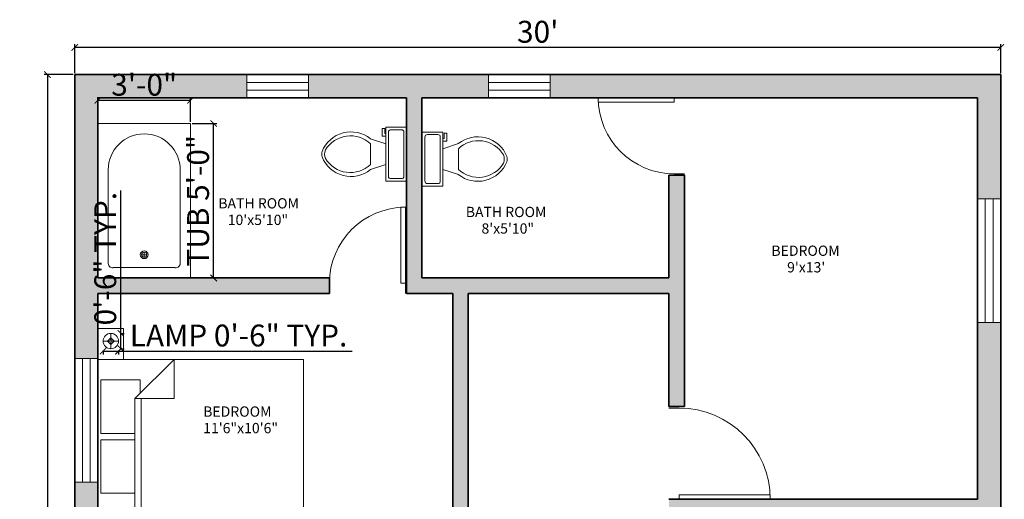
# Model space of a CAD drawing. Units: inches. Extents: x 3799 to 20199, y 1682 to 8087.
# Tile 17 of 30: x 10500 to 10883, y 7631 to 7817. Entities that reach past the tile are written whole.
import ezdxf

# ---------------------------------------------------------------- set-up
doc = ezdxf.new("R2010")
doc.units = ezdxf.units.IN
for name, color, linetype, lineweight in [('A-ANNO-DIMS', 2, 'Continuous', 18), ('A-AREA-IDEN', 7, 'Continuous', 18), ('A-DOOR', 3, 'Continuous', 18), ('A-FLOR-FIXT', 9, 'Continuous', 18), ('A-FURN', 8, 'Continuous', 18), ('A-GLAZ', 152, 'Continuous', 18), ('A-WALL', 7, 'Continuous', 35), ('A-WALL-PATT', 252, 'Continuous', 13)]:
    doc.layers.add(name, color=color, linetype=linetype, lineweight=lineweight)
doc.styles.get("Standard").update_dxf_attribs({"font": 'arial.ttf'})
doc.dimstyles.new('ISO-25', dxfattribs={"dimtxt": 8.5, "dimasz": 2.5, "dimexe": 1.25, "dimexo": 0.625, "dimtad": 1, "dimdec": 0, "dimlunit": 3, "dimtxsty": 'Standard', "dimblk": 'ARCHTICK', "dimcen": 2.5, "dimadec": 0, "dimazin": 0, "dimtfac": 1, "dimtdec": 0, "dimtmove": 0, "dimatfit": 3, "dimfxl": 1, "dimarcsym": 0})

# ---------------------------------------------------------------- blocks, each defined once
blk = doc.blocks.new('*U48')
for p, q in [((-750, 0), (-750, -100)), ((0, 0), (0, -100))]:
    blk.add_line(p, q)
blk.add_lwpolyline([(0, 0), (0, 750), (-43.75, 750), (-43.75, 0)], close=True)
blk.add_arc((0, 0), 750, 90, 180)
blk = doc.blocks.new('*U124')
for p, q in [((0, 0), (0, -100)), ((-900, 0), (-900, -100))]:
    blk.add_line(p, q)
blk.add_lwpolyline([(0, 0), (0, 900), (-43.75, 900), (-43.75, 0)], close=True)
blk.add_arc((0, 0), 900, 90, 180)
blk = doc.blocks.new('Bed - Queen')
for p, q in [((0, -80.00003), (0, 0)), ((0, 0), (59.99999, 0)), ((59.99999, 0), (59.99999, -80.00003)), ((7.99999, -1.2), (28.79998, -1.2)), ((7.99999, -14.4), (7.99999, -1.2)), ((28.79998, -1.2), (28.79998, -14.4)), ((31.19999, -1.2), (51.99999, -1.2)), ((31.19999, -14.4), (31.19999, -1.2)), ((51.99999, -1.2), (51.99999, -16.4)), ((0, -14.4), (44.8, -14.4)), ((59.99999, -29.6), (44.8, -14.4)), ((44.8, -14.4), (44.8, -29.6)), ((44.8, -16.8), (0, -16.8)), ((51.99999, -16.4), (46.79936, -16.4)), ((44.8, -29.6), (59.99999, -29.6)), ((59.99999, -80.00003), (0, -80.00003))]:
    blk.add_line(p, q)
blk = doc.blocks.new('Lamp - Table')
for p, q in [((-1, 0), (-7, 0)), ((0, 3), (-3, 0)), ((-3, 0), (0, -3)), ((0, 7), (0, 1)), ((3, 0), (0, 3)), ((0, -3), (3, 0)), ((1, 0), (7, 0)), ((0, -1), (0, -7))]:
    blk.add_line(p, q)
for radius in [7, 1]:
    blk.add_circle((0, 0), radius)
blk = doc.blocks.new('Bath Tub - 26 x 60 in.')
for p, q in [((8, -18), (10, -18)), ((9, -17), (9, -19))]:
    blk.add_line(p, q)
blk.add_lwpolyline([(0, -36), (0, 0), (60, 0), (60, -36)], close=True)
for points in [[(4, -30), (4, -6)], [(6, -4), (42, -4)], [(42, -32), (6, -32)]]:
    blk.add_lwpolyline(points)
for radius in [1.5, 1]:
    blk.add_circle((9, -18), radius)
for centre, radius, start, end in [((5.75, -5.75), 1.77, 81.8699, 188.1301), ((42, -18), 14, 270, 90), ((5.75, -30.25), 1.77, 171.8699, 278.1301)]:
    blk.add_arc(centre, radius, start, end)
blk = doc.blocks.new('Toilet - top')
for p, q in [((9.5, -6), (9.5, -2)), ((-10, -8.5), (-8, -8.5)), ((-10, -9.5), (-10, -8.5)), ((-7, -9.5), (-10, -9.5)), ((-8, -8.5), (-8, -8)), ((-7, -8), (-7, -9.5)), ((-4, -8), (-6, -14)), ((4, -8), (6, -14)), ((4, -14), (-4, -14))]:
    blk.add_line(p, q)
blk.add_lwpolyline([(10.5, -8), (10.5, 0), (-10.5, 0), (-10.5, -8)], close=True)
for points in [[(-9.5, -2), (-9.5, -6)], [(8.5, -1), (-8.5, -1)], [(-8.5, -7), (8.5, -7)]]:
    blk.add_lwpolyline(points)
for centre, radius, start, end in [((-8.62, -1.88), 0.884, 81.8699, 188.1301), ((8.62, -1.88), 0.884, 351.8699, 98.1301), ((-8.62, -6.12), 0.884, 171.8699, 278.1301), ((8.62, -6.12), 0.884, 261.8699, 8.1301), ((3.52, -21.58), 12.17, 141.4691, 247.9714), ((4.2, -21.82), 11.33, 136.3677, 238.9468), ((-3.52, -21.58), 12.17, 292.0284, 38.5307), ((-4.2, -21.82), 11.33, 301.053, 43.6321), ((0, -27.88), 4, 245.7318, 294.2682), ((0, -29), 4, 254.8605, 285.1395)]:
    blk.add_arc(centre, radius, start, end)
blk = doc.blocks.new('_ArchTick')
at = {"color": 0, "linetype": 'ByBlock', "const_width": 0.15}
blk.add_lwpolyline([(-0.5, -0.5), (0.5, 0.5)], dxfattribs=at)
blk = doc.blocks.new('*D175')
at = {"layer": 'A-ANNO-DIMS', "color": 0, "lineweight": -2, "transparency": 16777216}
for p, q in [((10521.87, 7796.25), (10521.87, 7807.45)), ((10881.87, 7806.2), (10521.87, 7806.2)), ((10881.87, 7796.25), (10881.87, 7807.45))]:
    blk.add_line(p, q, dxfattribs=at)
at = {"layer": 'Defpoints', "color": 0, "transparency": 16777216}
for p in [(10521.87, 7806.2), (10521.87, 7795.62), (10881.87, 7795.62)]:
    blk.add_point(p, dxfattribs=at)
at = {"layer": 'A-ANNO-DIMS', "color": 0, "lineweight": -2, "transparency": 16777216, "xscale": 2.5, "yscale": 2.5, "zscale": 2.5, "rotation": 180}
blk.add_blockref('_ArchTick', (10521.87, 7806.2), dxfattribs=at)
at = {"layer": 'A-ANNO-DIMS', "color": 0, "lineweight": -2, "transparency": 16777216, "xscale": 2.5, "yscale": 2.5, "zscale": 2.5}
blk.add_blockref('_ArchTick', (10881.87, 7806.2), dxfattribs=at)
at = {"layer": 'A-ANNO-DIMS', "color": 0, "transparency": 16777216, "insert": (10701.87, 7811.17), "char_height": 8.5, "attachment_point": 5}
blk.add_mtext("30'", dxfattribs=at)
blk = doc.blocks.new('*D176')
at = {"layer": 'A-ANNO-DIMS', "color": 0, "lineweight": -2, "transparency": 16777216}
for p, q in [((10521.25, 7795.62), (10509.98, 7795.62)), ((10511.23, 7795.62), (10511.23, 7315.62)), ((10521.25, 7315.62), (10509.98, 7315.62))]:
    blk.add_line(p, q, dxfattribs=at)
at = {"layer": 'Defpoints', "color": 0, "transparency": 16777216}
for p in [(10521.87, 7795.62), (10511.23, 7315.62), (10521.87, 7315.62)]:
    blk.add_point(p, dxfattribs=at)
at = {"layer": 'A-ANNO-DIMS', "color": 0, "lineweight": -2, "transparency": 16777216, "xscale": 2.5, "yscale": 2.5, "zscale": 2.5}
for p, rotation in [((10511.23, 7795.62), 90), ((10511.23, 7315.62), 270)]:
    blk.add_blockref('_ArchTick', p, dxfattribs=dict(at, rotation=rotation))
at = {"layer": 'A-ANNO-DIMS', "color": 0, "transparency": 16777216, "insert": (10506.27, 7555.62), "char_height": 8.5, "attachment_point": 5, "rotation": 90}
blk.add_mtext("40'", dxfattribs=at)
blk = doc.blocks.new('WIN-24IN-9IN-FRAME')
for p, q in [((0, 24), (9, 24)), ((3, 0), (3, 24)), ((6, 0), (6, 24)), ((0, 0), (9, 0))]:
    blk.add_line(p, q)
blk = doc.blocks.new('WIN-48IN-9IN-FRAME')
for p, q in [((0, 0), (0, 9)), ((48, 0), (48, 9)), ((48, 6), (0, 6)), ((48, 3), (0, 3))]:
    blk.add_line(p, q)
blk = doc.blocks.new('*D250')
at = {"layer": 'A-ANNO-DIMS', "color": 0, "lineweight": -2, "transparency": 16777216}
for p, q in [((10532.9, 7688.46), (10532.9, 7686.94)), ((10532.9, 7688.19), (10538.9, 7688.19)), ((10538.9, 7688.46), (10538.9, 7686.94)), ((10538.9, 7688.19), (10629.72, 7688.19))]:
    blk.add_line(p, q, dxfattribs=at)
at = {"layer": 'Defpoints', "color": 0, "transparency": 16777216}
for p in [(10532.9, 7689.09), (10538.9, 7689.09), (10538.9, 7688.19)]:
    blk.add_point(p, dxfattribs=at)
at = {"layer": 'A-ANNO-DIMS', "color": 0, "lineweight": -2, "transparency": 16777216, "xscale": 2.5, "yscale": 2.5, "zscale": 2.5, "rotation": 180}
blk.add_blockref('_ArchTick', (10532.9, 7688.19), dxfattribs=at)
at = {"layer": 'A-ANNO-DIMS', "color": 0, "lineweight": -2, "transparency": 16777216, "xscale": 2.5, "yscale": 2.5, "zscale": 2.5}
blk.add_blockref('_ArchTick', (10538.9, 7688.19), dxfattribs=at)
at = {"layer": 'A-ANNO-DIMS', "color": 0, "transparency": 16777216, "insert": (10585.56, 7693.15), "char_height": 8.5, "attachment_point": 5}
blk.add_mtext('LAMP 0\'-6" TYP.', dxfattribs=at)
blk = doc.blocks.new('*D251')
at = {"layer": 'A-ANNO-DIMS', "color": 0, "lineweight": -2, "transparency": 16777216}
for p, q in [((10539.8, 7695.09), (10539.8, 7750.65)), ((10539.52, 7695.09), (10541.05, 7695.09)), ((10539.8, 7689.09), (10539.8, 7695.09)), ((10539.52, 7689.09), (10541.05, 7689.09))]:
    blk.add_line(p, q, dxfattribs=at)
at = {"layer": 'Defpoints', "color": 0, "transparency": 16777216}
for p in [(10538.9, 7695.09), (10539.8, 7695.09), (10538.9, 7689.09)]:
    blk.add_point(p, dxfattribs=at)
at = {"layer": 'A-ANNO-DIMS', "color": 0, "lineweight": -2, "transparency": 16777216, "xscale": 2.5, "yscale": 2.5, "zscale": 2.5}
for p, rotation in [((10539.8, 7695.09), 90), ((10539.8, 7689.09), 270)]:
    blk.add_blockref('_ArchTick', p, dxfattribs=dict(at, rotation=rotation))
at = {"layer": 'A-ANNO-DIMS', "color": 0, "transparency": 16777216, "insert": (10534.83, 7724.12), "char_height": 8.5, "attachment_point": 5, "rotation": 90}
blk.add_mtext('0\'-6" TYP.', dxfattribs=at)
blk = doc.blocks.new('*D308')
at = {"layer": 'A-ANNO-DIMS', "color": 0, "lineweight": -2, "transparency": 16777216}
for p, q in [((10567.5, 7776.62), (10577.12, 7776.62)), ((10575.87, 7716.62), (10575.87, 7776.62)), ((10567.5, 7716.62), (10577.12, 7716.62))]:
    blk.add_line(p, q, dxfattribs=at)
at = {"layer": 'Defpoints', "color": 0, "transparency": 16777216}
for p in [(10566.87, 7776.62), (10575.87, 7776.62), (10566.87, 7716.62)]:
    blk.add_point(p, dxfattribs=at)
at = {"layer": 'A-ANNO-DIMS', "color": 0, "lineweight": -2, "transparency": 16777216, "xscale": 2.5, "yscale": 2.5, "zscale": 2.5}
for p, rotation in [((10575.87, 7776.62), 90), ((10575.87, 7716.62), 270)]:
    blk.add_blockref('_ArchTick', p, dxfattribs=dict(at, rotation=rotation))
at = {"layer": 'A-ANNO-DIMS', "color": 0, "transparency": 16777216, "insert": (10570.91, 7746.62), "char_height": 8.5, "attachment_point": 5, "rotation": 90}
blk.add_mtext('TUB 5\'-0"', dxfattribs=at)
blk = doc.blocks.new('*D309')
at = {"layer": 'A-ANNO-DIMS', "color": 0, "lineweight": -2, "transparency": 16777216}
for p, q in [((10530.87, 7777.25), (10530.87, 7786.87)), ((10566.87, 7777.25), (10566.87, 7786.87)), ((10566.87, 7785.62), (10530.87, 7785.62))]:
    blk.add_line(p, q, dxfattribs=at)
at = {"layer": 'Defpoints', "color": 0, "transparency": 16777216}
for p in [(10530.87, 7785.62), (10530.87, 7776.62), (10566.87, 7776.62)]:
    blk.add_point(p, dxfattribs=at)
at = {"layer": 'A-ANNO-DIMS', "color": 0, "lineweight": -2, "transparency": 16777216, "xscale": 2.5, "yscale": 2.5, "zscale": 2.5, "rotation": 180}
blk.add_blockref('_ArchTick', (10530.87, 7785.62), dxfattribs=at)
at = {"layer": 'A-ANNO-DIMS', "color": 0, "lineweight": -2, "transparency": 16777216, "xscale": 2.5, "yscale": 2.5, "zscale": 2.5}
blk.add_blockref('_ArchTick', (10566.87, 7785.62), dxfattribs=at)
at = {"layer": 'A-ANNO-DIMS', "color": 0, "transparency": 16777216, "insert": (10548.87, 7790.59), "char_height": 8.5, "attachment_point": 5}
blk.add_mtext('3\'-0"', dxfattribs=at)

msp = doc.modelspace()

# ---------------------------------------------------------------- hatches: boundary and pattern name
at = {"layer": 'A-WALL-PATT'}
h = msp.add_hatch(color=256, dxfattribs=at)
h.dxf.hatch_style = 1
h.paths.add_polyline_path([(10588.75, 7795.62), (10521.87, 7795.62), (10521.87, 7685.33), (10530.87, 7685.33), (10530.87, 7696.98), (10530.87, 7710.62), (10620.87, 7710.62), (10620.87, 7716.62), (10530.87, 7716.62), (10530.87, 7786.62), (10588.75, 7786.62)])
h.paths.add_polyline_path([(10682.68, 7795.62), (10612.75, 7795.62), (10612.75, 7786.62), (10650.87, 7786.62), (10650.87, 7716.62), (10650.87, 7710.62), (10668.87, 7710.62), (10668.87, 7620.62), (10674.87, 7620.62), (10674.87, 7710.62), (10752.87, 7710.62), (10752.87, 7666.62), (10758.87, 7666.62), (10758.87, 7756.62), (10752.87, 7756.62), (10752.87, 7716.62), (10656.87, 7716.62), (10656.87, 7786.62), (10682.68, 7786.62)])
h.paths.add_polyline_path([(10881.87, 7795.62), (10706.68, 7795.62), (10706.68, 7786.62), (10752.87, 7786.62), (10758.87, 7786.62), (10872.87, 7786.62), (10872.87, 7747.36), (10881.87, 7747.36)])
h.paths.add_polyline_path([(10881.87, 7699.36), (10872.87, 7699.36), (10872.87, 7630.62), (10752.87, 7630.62), (10752.87, 7624.62), (10872.87, 7624.62), (10872.87, 7608.58), (10881.87, 7608.58)])
h.paths.add_polyline_path([(10674.87, 7584.62), (10530.87, 7584.62), (10530.87, 7637.33), (10521.87, 7637.33), (10521.87, 7550.27), (10530.87, 7550.27), (10530.87, 7578.62), (10626.87, 7578.62), (10626.87, 7526.73), (10632.87, 7526.73), (10632.87, 7578.62), (10674.87, 7578.62)])
h.paths.add_polyline_path([(10530.87, 7488.62), (10632.87, 7488.62), (10632.87, 7496.73), (10628.93, 7496.73), (10626.87, 7496.73), (10626.87, 7494.62), (10530.87, 7494.62), (10530.87, 7526.27), (10521.87, 7526.27), (10521.87, 7458.64), (10530.87, 7458.64)])
h.paths.add_polyline_path([(10656.87, 7494.62), (10632.87, 7494.62), (10632.87, 7488.62), (10656.87, 7488.62)])
h.paths.add_polyline_path([(10530.87, 7434.64), (10521.87, 7434.64), (10521.87, 7400.54), (10530.87, 7400.54), (10530.87, 7404.62), (10704.87, 7404.62), (10704.87, 7410.62), (10530.87, 7410.62)])
h.paths.add_polyline_path([(10745.87, 7404.62), (10763.75, 7404.62), (10763.75, 7410.62), (10740.87, 7410.62), (10740.87, 7315.62), (10789.88, 7315.62), (10789.88, 7324.62), (10745.87, 7324.62)])
h.paths.add_polyline_path([(10881.87, 7429.64), (10872.87, 7429.64), (10872.87, 7408.03), (10872.87, 7324.62), (10849.88, 7324.62), (10849.88, 7315.62), (10881.87, 7315.62)])
h.paths.add_polyline_path([(10881.87, 7560.58), (10872.87, 7560.58), (10872.87, 7468.62), (10758.87, 7468.62), (10758.87, 7588.62), (10752.87, 7588.62), (10752.87, 7462.62), (10872.87, 7462.62), (10872.87, 7453.64), (10881.87, 7453.64)])

# ---------------------------------------------------------------- linework, layer by layer
at = {"layer": 'A-FURN'}
msp.add_lwpolyline([(10530.87, 7684.98), (10540.87, 7684.98), (10540.87, 7696.98), (10530.87, 7696.98)], close=True, dxfattribs=at)
at = {"layer": 'A-WALL'}
for p, q in [((10881.87, 7795.62), (10521.87, 7795.62)), ((10521.87, 7795.62), (10521.87, 7315.62)), ((10881.87, 7315.62), (10881.87, 7795.62)), ((10530.87, 7786.62), (10530.87, 7716.62)), ((10650.87, 7786.62), (10530.87, 7786.62)), ((10650.87, 7786.62), (10650.87, 7716.62)), ((10656.87, 7786.62), (10656.87, 7716.62)), ((10752.87, 7786.62), (10656.87, 7786.62)), ((10752.87, 7786.62), (10758.87, 7786.62)), ((10872.87, 7786.62), (10758.87, 7786.62)), ((10872.87, 7630.62), (10872.87, 7786.62)), ((10752.87, 7756.62), (10752.87, 7716.62)), ((10752.87, 7756.62), (10758.87, 7756.62)), ((10758.87, 7756.62), (10758.87, 7666.62)), ((10620.87, 7716.62), (10530.87, 7716.62)), ((10620.87, 7716.62), (10620.87, 7710.62)), ((10650.87, 7716.62), (10650.87, 7710.62)), ((10752.87, 7716.62), (10656.87, 7716.62)), ((10530.87, 7710.62), (10530.87, 7584.62)), ((10620.87, 7710.62), (10530.87, 7710.62)), ((10668.87, 7710.62), (10650.87, 7710.62)), ((10668.87, 7710.62), (10668.87, 7620.62)), ((10752.87, 7710.62), (10674.87, 7710.62)), ((10674.87, 7710.62), (10674.87, 7620.62)), ((10752.87, 7710.62), (10752.87, 7666.62)), ((10758.87, 7666.62), (10752.87, 7666.62)), ((10872.87, 7630.62), (10752.87, 7630.62))]:
    msp.add_line(p, q, dxfattribs=at)

# ---------------------------------------------------------------- block references
at = {"layer": 'A-DOOR', "xscale": 0.0393700787401575, "yscale": 0.0393700787401575, "zscale": 0.0393700787401575}
for name, p, rotation in [('*U48', (10754.93, 7786.62), 90), ('*U124', (10756.81, 7630.62), 270)]:
    msp.add_blockref(name, p, dxfattribs=dict(at, rotation=rotation))
msp.add_blockref('*U48', (10650.4, 7714.56), dxfattribs=at)
at = {"layer": 'A-FLOR-FIXT'}
for name, p, rotation in [('Bath Tub - 26 x 60 in.', (10530.87, 7716.62), 90), ('Toilet - top', (10650.87, 7764.7), 270)]:
    msp.add_blockref(name, p, dxfattribs=dict(at, rotation=rotation))
at = {"layer": 'A-FLOR-FIXT', "xscale": -1, "rotation": 90}
msp.add_blockref('Toilet - top', (10657, 7762.82), dxfattribs=at)
at = {"layer": 'A-FURN', "xscale": 0.4285713367347382, "yscale": 0.4285713367347382, "zscale": 0.4285713367347382}
msp.add_blockref('Lamp - Table', (10535.9, 7692.09), dxfattribs=at)
at = {"layer": 'A-FURN', "rotation": 90}
msp.add_blockref('Bed - Queen', (10530.87, 7624.98), dxfattribs=at)
at = {"layer": 'A-GLAZ', "rotation": 90}
for name, p in [('WIN-24IN-9IN-FRAME', (10612.75, 7786.62)), ('WIN-24IN-9IN-FRAME', (10706.68, 7786.62)), ('WIN-48IN-9IN-FRAME', (10881.87, 7699.36)), ('WIN-48IN-9IN-FRAME', (10530.87, 7637.33))]:
    msp.add_blockref(name, p, dxfattribs=at)

# ---------------------------------------------------------------- texts
at = {"layer": 'A-AREA-IDEN'}
for s, p in [('BATH ROOM', (10577.68, 7743.62)), ('BATH ROOM', (10673.89, 7740.26)), ('   10\'x5\'10"', (10577.68, 7737.19)), ('     8\'x5\'10"', (10673.89, 7733.84)), ('BEDROOM', (10792.7, 7725.2)), ("     9'x13'", (10792.7, 7718.77)), ('BEDROOM', (10571.81, 7662.71)), ('11\'6"x10\'6"', (10571.81, 7656.29))]:
    msp.add_text(s, height=4, rotation=0.0008, dxfattribs=at).set_placement(p)

# ---------------------------------------------------------------- dimensions: what is measured, and where the dimension line sits
at = {"layer": 'A-ANNO-DIMS'}
dim = msp.add_linear_dim(base=(10521.87, 7806.2), p1=(10881.87, 7795.62), p2=(10521.87, 7795.62), dimstyle='ISO-25', override={"dimclrd": 0, "dimclre": 0, "dimclrt": 0}, dxfattribs=at)
dim.commit()
dim.dimension.update_dxf_attribs({"geometry": '*D175', "text_midpoint": (10701.87, 7811.17)})
for base, p1, p2, angle, override, picture, middle in [((10511.23, 7315.62), (10521.87, 7795.62), (10521.87, 7315.62), 90, {"dimclrd": 0, "dimclre": 0, "dimclrt": 0}, '*D176', (10506.27, 7555.62)), ((10530.87, 7785.62), (10566.87, 7776.62), (10530.87, 7776.62), 180, {"dimdec": 1, "dimlfac": 1, "dimrnd": 0, "dimzin": 1, "dimdsep": 46, "dimlunit": 4, "dimfrac": 2}, '*D309', (10548.87, 7790.59))]:
    dim = msp.add_linear_dim(base=base, p1=p1, p2=p2, angle=angle, dimstyle='ISO-25', override=override, dxfattribs=at)
    dim.commit()
    dim.dimension.update_dxf_attribs({"geometry": picture, "text_midpoint": middle})
for base, p1, p2, text, picture, middle in [((10575.87, 7776.62), (10566.87, 7716.62), (10566.87, 7776.62), 'TUB <>', '*D308', (10570.91, 7746.62)), ((10539.8, 7695.09), (10538.9, 7689.09), (10538.9, 7695.09), '<> TYP.', '*D251', (10534.83, 7724.12))]:
    dim = msp.add_linear_dim(base=base, p1=p1, p2=p2, angle=90, text=text, dimstyle='ISO-25', override={"dimdec": 1, "dimlfac": 1, "dimrnd": 0, "dimzin": 1, "dimdsep": 46, "dimlunit": 4, "dimfrac": 2}, dxfattribs=at)
    dim.commit()
    dim.dimension.update_dxf_attribs({"geometry": picture, "text_midpoint": middle})
dim = msp.add_linear_dim(base=(10538.9, 7688.19), p1=(10532.9, 7689.09), p2=(10538.9, 7689.09), text='LAMP <> TYP.', dimstyle='ISO-25', override={"dimdec": 1, "dimlfac": 1, "dimrnd": 0, "dimzin": 1, "dimdsep": 46, "dimlunit": 4, "dimfrac": 2}, dxfattribs=at)
dim.commit()
dim.dimension.update_dxf_attribs({"geometry": '*D250', "text_midpoint": (10585.56, 7693.15)})

doc.saveas('drawing.dxf')
